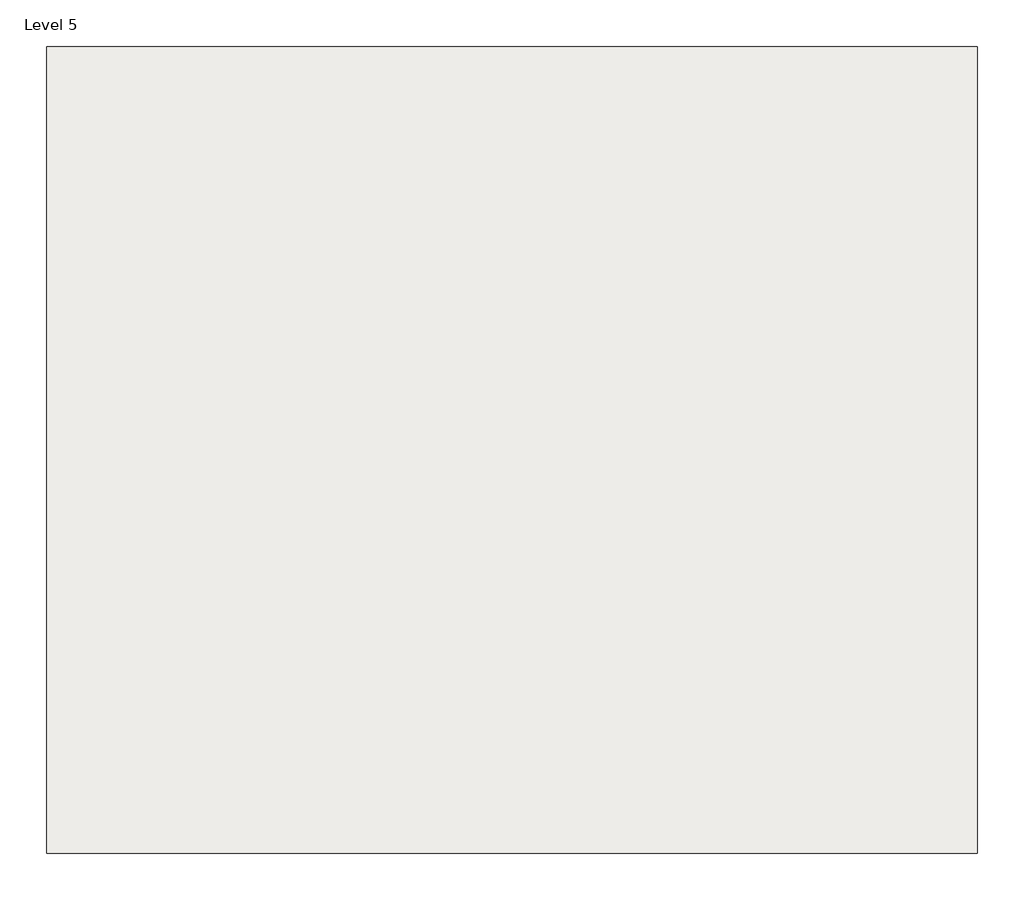
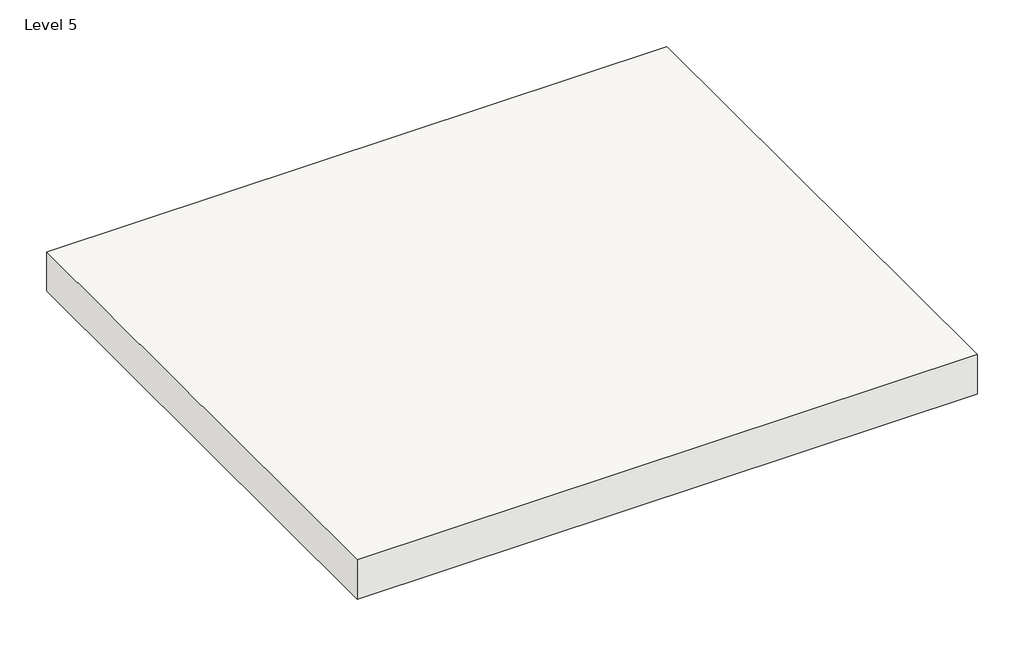
# One storey: 1 roof.
"""IFC4 building model written with IfcOpenShell, lengths in millimetres."""

from ifc_helpers import new_model, si_unit, frame, origin, place, context, project, spatial, polyline, outline, extrude, element, save

model = new_model("IFC4")

# Units and contexts
model_context = context("Model", 3, world=origin())
ifc_project = project(units=[si_unit("LENGTHUNIT", "METRE", prefix="MILLI")], contexts=[model_context])

# Site, building, storey
site = spatial("IfcSite", under=ifc_project)
building = spatial("IfcBuilding", under=site)
storey = spatial("IfcBuildingStorey", under=building, Name="Level 5", Elevation=12192.0)

# Roof
placement = place(None, origin())
element("IfcRoof", 1, ObjectType="Generic - 12\"", at=placement, inside=storey, context=model_context, shape_type="SweptSolid", body=[
    extrude(outline(polyline([(-6072.0950764, -10413.9173218), (-6072.0950764, -14376.3173218), (-10644.0950764, -14376.3173218), (-10644.0950764, -10413.9173218), (-6072.0950764, -10413.9173218)])), frame((0.0, 0.0, 12192.0), z_axis=(0.0, 0.0, 1.0), x_axis=(1.0, 0.0, 0.0)), (0.0, 0.0, 1.0), 304.8),
])

save(model, "model.ifc")

# Revit data of these elements
# Type "Generic - 12\""
#   Assembly Code = "B1020"
#   Layers, outside or top first: 1' - 0" no material (function 1)
# Element 1 (IfcRoof, "Generic - 12\"")
#   built-in parameter 1001705 = 41 (stored number, unit not read)
#   built-in parameter 1001710 = 33615
#   Phase Created = New Construction
#   Materials on its faces: "Default Roof"
# Materials
#   "Default Roof": colour RGB 88 101 114, transparency 0, Cost = 0
